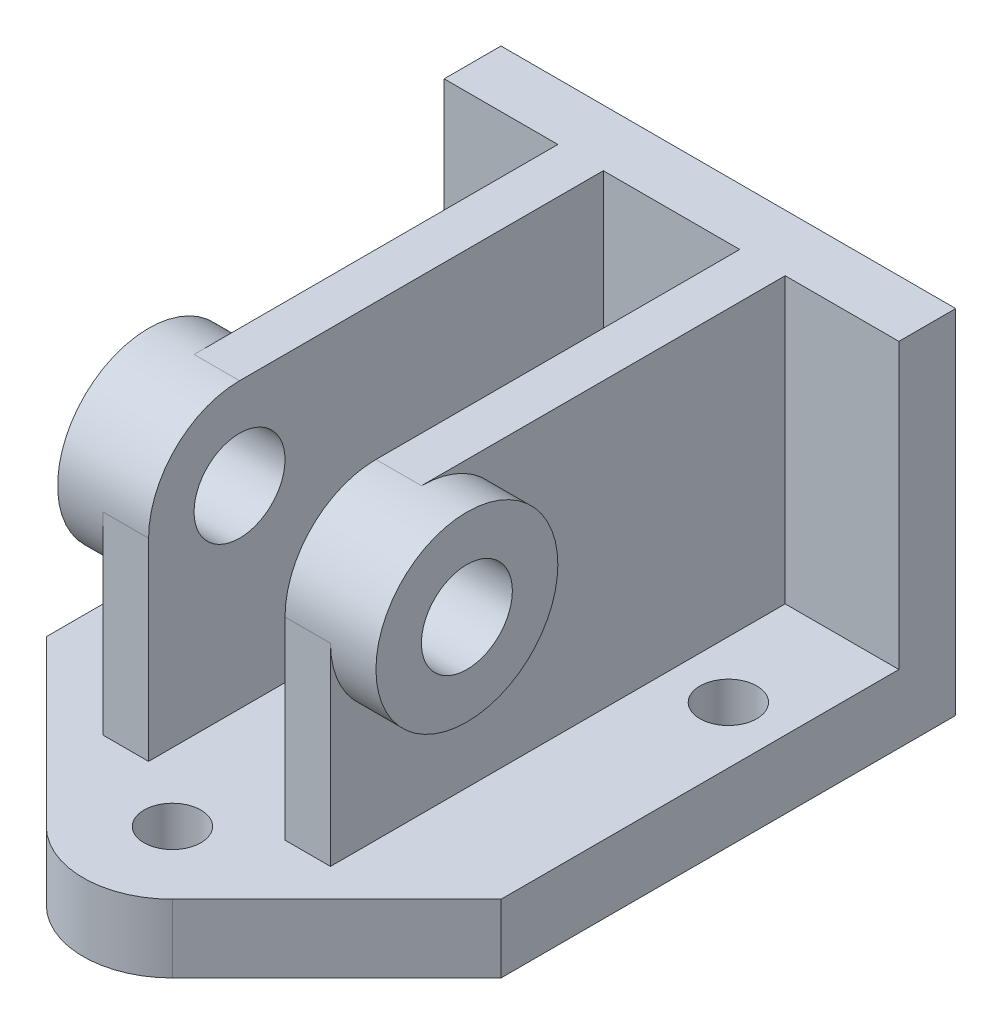
ISO-10303-21;
HEADER;
FILE_DESCRIPTION(('STEP AP214'),'2;1');
FILE_NAME('part.step','',(''),(''),'','','');
FILE_SCHEMA(('AUTOMOTIVE_DESIGN { 1 0 10303 214 1 1 1 1 }'));
ENDSEC;
DATA;
#1=APPLICATION_CONTEXT('core data for automotive mechanical design processes');
#2=APPLICATION_PROTOCOL_DEFINITION('international standard','automotive_design',2000,#1);
#3=PRODUCT_CONTEXT('',#1,'mechanical');
#4=PRODUCT('Part','Part','',(#3));
#5=PRODUCT_RELATED_PRODUCT_CATEGORY('part','',(#4));
#6=PRODUCT_DEFINITION_FORMATION('','',#4);
#7=PRODUCT_DEFINITION_CONTEXT('part definition',#1,'design');
#8=PRODUCT_DEFINITION('design','',#6,#7);
#9=PRODUCT_DEFINITION_SHAPE('','',#8);
#10=(LENGTH_UNIT() NAMED_UNIT(*) SI_UNIT(.MILLI.,.METRE.));
#11=(NAMED_UNIT(*) PLANE_ANGLE_UNIT() SI_UNIT($,.RADIAN.));
#12=(NAMED_UNIT(*) SI_UNIT($,.STERADIAN.) SOLID_ANGLE_UNIT());
#13=UNCERTAINTY_MEASURE_WITH_UNIT(LENGTH_MEASURE(1.E-05),#10,'distance_accuracy_value','');
#14=(GEOMETRIC_REPRESENTATION_CONTEXT(3) GLOBAL_UNCERTAINTY_ASSIGNED_CONTEXT((#13)) GLOBAL_UNIT_ASSIGNED_CONTEXT((#10,
#11,#12)) REPRESENTATION_CONTEXT('',''));
#15=CARTESIAN_POINT('',(0.,0.,0.));
#16=DIRECTION('',(0.,0.,1.));
#17=DIRECTION('',(1.,0.,0.));
#18=AXIS2_PLACEMENT_3D('',#15,#16,#17);
#19=CARTESIAN_POINT('',(-6.,31.,5.));
#20=DIRECTION('',(-1.,0.,0.));
#21=DIRECTION('',(0.,0.,1.));
#22=AXIS2_PLACEMENT_3D('',#19,#20,#21);
#23=PLANE('',#22);
#24=DIRECTION('',(0.,0.,-1.));
#25=VECTOR('',#24,1.);
#26=CARTESIAN_POINT('',(-6.,31.,5.));
#27=LINE('',#26,#25);
#28=CARTESIAN_POINT('',(-5.99999999999999,31.,37.));
#29=VERTEX_POINT('',#28);
#30=CARTESIAN_POINT('',(-6.,31.,5.));
#31=VERTEX_POINT('',#30);
#32=EDGE_CURVE('E289',#29,#31,#27,.T.);
#33=ORIENTED_EDGE('',*,*,#32,.F.);
#34=CARTESIAN_POINT('',(-5.99999999999999,23.,37.));
#35=DIRECTION('',(-1.,0.,0.));
#36=DIRECTION('',(0.,0.,1.));
#37=AXIS2_PLACEMENT_3D('',#34,#35,#36);
#38=CIRCLE('',#37,7.99999999999999);
#39=CARTESIAN_POINT('',(-5.99999999999999,23.,45.));
#40=VERTEX_POINT('',#39);
#41=EDGE_CURVE('E172',#29,#40,#38,.F.);
#42=ORIENTED_EDGE('',*,*,#41,.T.);
#43=DIRECTION('',(0.,-1.,0.));
#44=VECTOR('',#43,1.);
#45=CARTESIAN_POINT('',(-5.99999999999999,31.,45.));
#46=LINE('',#45,#44);
#47=CARTESIAN_POINT('',(-5.99999999999999,6.,45.));
#48=VERTEX_POINT('',#47);
#49=EDGE_CURVE('E168',#40,#48,#46,.T.);
#50=ORIENTED_EDGE('',*,*,#49,.T.);
#51=DIRECTION('',(0.,0.,-1.));
#52=VECTOR('',#51,1.);
#53=CARTESIAN_POINT('',(-6.,6.,5.));
#54=LINE('',#53,#52);
#55=CARTESIAN_POINT('',(-6.,6.,5.));
#56=VERTEX_POINT('',#55);
#57=EDGE_CURVE('E306',#48,#56,#54,.T.);
#58=ORIENTED_EDGE('',*,*,#57,.T.);
#59=DIRECTION('',(0.,-1.,0.));
#60=VECTOR('',#59,1.);
#61=CARTESIAN_POINT('',(-6.,31.,5.));
#62=LINE('',#61,#60);
#63=EDGE_CURVE('E189',#31,#56,#62,.T.);
#64=ORIENTED_EDGE('',*,*,#63,.F.);
#65=EDGE_LOOP('',(#33,#42,#50,#58,#64));
#66=FACE_BOUND('',#65,.T.);
#67=CARTESIAN_POINT('',(-5.99999999999999,23.,37.));
#68=DIRECTION('',(-1.,0.,0.));
#69=DIRECTION('',(0.,0.,1.));
#70=AXIS2_PLACEMENT_3D('',#67,#68,#69);
#71=CIRCLE('',#70,4.);
#72=CARTESIAN_POINT('',(-5.99999999999999,23.,41.));
#73=VERTEX_POINT('',#72);
#74=EDGE_CURVE('E354',#73,#73,#71,.T.);
#75=ORIENTED_EDGE('',*,*,#74,.T.);
#76=EDGE_LOOP('',(#75));
#77=FACE_BOUND('',#76,.T.);
#78=ADVANCED_FACE('F39',(#66,#77),#23,.F.);
#79=CARTESIAN_POINT('',(6.,31.,5.));
#80=DIRECTION('',(1.,0.,0.));
#81=DIRECTION('',(0.,0.,-1.));
#82=AXIS2_PLACEMENT_3D('',#79,#80,#81);
#83=PLANE('',#82);
#84=CARTESIAN_POINT('',(6.00000000000001,23.,37.));
#85=DIRECTION('',(1.,0.,0.));
#86=DIRECTION('',(0.,0.,-1.));
#87=AXIS2_PLACEMENT_3D('',#84,#85,#86);
#88=CIRCLE('',#87,7.99999999999999);
#89=CARTESIAN_POINT('',(6.,31.,37.));
#90=VERTEX_POINT('',#89);
#91=CARTESIAN_POINT('',(6.00000000000001,23.,45.));
#92=VERTEX_POINT('',#91);
#93=EDGE_CURVE('E349',#90,#92,#88,.T.);
#94=ORIENTED_EDGE('',*,*,#93,.F.);
#95=DIRECTION('',(0.,0.,1.));
#96=VECTOR('',#95,1.);
#97=CARTESIAN_POINT('',(6.,31.,5.));
#98=LINE('',#97,#96);
#99=CARTESIAN_POINT('',(6.,31.,5.));
#100=VERTEX_POINT('',#99);
#101=EDGE_CURVE('E295',#100,#90,#98,.T.);
#102=ORIENTED_EDGE('',*,*,#101,.F.);
#103=DIRECTION('',(0.,-1.,0.));
#104=VECTOR('',#103,1.);
#105=CARTESIAN_POINT('',(6.,31.,5.));
#106=LINE('',#105,#104);
#107=CARTESIAN_POINT('',(6.,6.,5.));
#108=VERTEX_POINT('',#107);
#109=EDGE_CURVE('E329',#100,#108,#106,.T.);
#110=ORIENTED_EDGE('',*,*,#109,.T.);
#111=DIRECTION('',(0.,0.,1.));
#112=VECTOR('',#111,1.);
#113=CARTESIAN_POINT('',(6.,6.,5.));
#114=LINE('',#113,#112);
#115=CARTESIAN_POINT('',(6.,6.,45.));
#116=VERTEX_POINT('',#115);
#117=EDGE_CURVE('E314',#108,#116,#114,.T.);
#118=ORIENTED_EDGE('',*,*,#117,.T.);
#119=DIRECTION('',(0.,-1.,0.));
#120=VECTOR('',#119,1.);
#121=CARTESIAN_POINT('',(6.,31.,45.));
#122=LINE('',#121,#120);
#123=EDGE_CURVE('E327',#92,#116,#122,.T.);
#124=ORIENTED_EDGE('',*,*,#123,.F.);
#125=EDGE_LOOP('',(#94,#102,#110,#118,#124));
#126=FACE_BOUND('',#125,.T.);
#127=CARTESIAN_POINT('',(6.00000000000001,23.,37.));
#128=DIRECTION('',(1.,0.,0.));
#129=DIRECTION('',(0.,0.,-1.));
#130=AXIS2_PLACEMENT_3D('',#127,#128,#129);
#131=CIRCLE('',#130,4.);
#132=CARTESIAN_POINT('',(6.00000000000001,23.,33.));
#133=VERTEX_POINT('',#132);
#134=EDGE_CURVE('E365',#133,#133,#131,.F.);
#135=ORIENTED_EDGE('',*,*,#134,.F.);
#136=EDGE_LOOP('',(#135));
#137=FACE_BOUND('',#136,.T.);
#138=ADVANCED_FACE('F347',(#126,#137),#83,.F.);
#139=CARTESIAN_POINT('',(6.,31.,45.));
#140=DIRECTION('',(0.,0.,-1.));
#141=DIRECTION('',(-1.,0.,0.));
#142=AXIS2_PLACEMENT_3D('',#139,#140,#141);
#143=PLANE('',#142);
#144=DIRECTION('',(1.,0.,0.));
#145=VECTOR('',#144,1.);
#146=CARTESIAN_POINT('',(-20.001,23.,45.));
#147=LINE('',#146,#145);
#148=CARTESIAN_POINT('',(10.,23.,45.));
#149=VERTEX_POINT('',#148);
#150=EDGE_CURVE('E369',#92,#149,#147,.T.);
#151=ORIENTED_EDGE('',*,*,#150,.F.);
#152=ORIENTED_EDGE('',*,*,#123,.T.);
#153=DIRECTION('',(1.,0.,0.));
#154=VECTOR('',#153,1.);
#155=CARTESIAN_POINT('',(6.,6.,45.));
#156=LINE('',#155,#154);
#157=CARTESIAN_POINT('',(10.,6.,45.));
#158=VERTEX_POINT('',#157);
#159=EDGE_CURVE('E320',#116,#158,#156,.T.);
#160=ORIENTED_EDGE('',*,*,#159,.T.);
#161=DIRECTION('',(0.,-1.,0.));
#162=VECTOR('',#161,1.);
#163=CARTESIAN_POINT('',(10.,31.,45.));
#164=LINE('',#163,#162);
#165=EDGE_CURVE('E326',#149,#158,#164,.T.);
#166=ORIENTED_EDGE('',*,*,#165,.F.);
#167=EDGE_LOOP('',(#151,#152,#160,#166));
#168=FACE_BOUND('',#167,.T.);
#169=ADVANCED_FACE('F390',(#168),#143,.F.);
#170=CARTESIAN_POINT('',(0.,31.,0.));
#171=DIRECTION('',(0.,1.,0.));
#172=DIRECTION('',(0.,0.,1.));
#173=AXIS2_PLACEMENT_3D('',#170,#171,#172);
#174=PLANE('',#173);
#175=DIRECTION('',(-1.,0.,0.));
#176=VECTOR('',#175,1.);
#177=CARTESIAN_POINT('',(20.001,31.,37.));
#178=LINE('',#177,#176);
#179=CARTESIAN_POINT('',(-10.,31.,37.));
#180=VERTEX_POINT('',#179);
#181=EDGE_CURVE('E174',#29,#180,#178,.T.);
#182=ORIENTED_EDGE('',*,*,#181,.F.);
#183=ORIENTED_EDGE('',*,*,#32,.T.);
#184=DIRECTION('',(1.,0.,0.));
#185=VECTOR('',#184,1.);
#186=CARTESIAN_POINT('',(-6.,31.,5.));
#187=LINE('',#186,#185);
#188=EDGE_CURVE('E288',#31,#100,#187,.T.);
#189=ORIENTED_EDGE('',*,*,#188,.T.);
#190=ORIENTED_EDGE('',*,*,#101,.T.);
#191=DIRECTION('',(1.,0.,0.));
#192=VECTOR('',#191,1.);
#193=CARTESIAN_POINT('',(-20.001,31.,37.));
#194=LINE('',#193,#192);
#195=CARTESIAN_POINT('',(10.,31.,37.));
#196=VERTEX_POINT('',#195);
#197=EDGE_CURVE('E348',#90,#196,#194,.T.);
#198=ORIENTED_EDGE('',*,*,#197,.T.);
#199=DIRECTION('',(0.,0.,-1.));
#200=VECTOR('',#199,1.);
#201=CARTESIAN_POINT('',(10.,31.,5.));
#202=LINE('',#201,#200);
#203=CARTESIAN_POINT('',(10.,31.,5.));
#204=VERTEX_POINT('',#203);
#205=EDGE_CURVE('E293',#196,#204,#202,.T.);
#206=ORIENTED_EDGE('',*,*,#205,.T.);
#207=DIRECTION('',(1.,0.,0.));
#208=VECTOR('',#207,1.);
#209=CARTESIAN_POINT('',(10.,31.,5.));
#210=LINE('',#209,#208);
#211=CARTESIAN_POINT('',(20.,31.,5.));
#212=VERTEX_POINT('',#211);
#213=EDGE_CURVE('E299',#204,#212,#210,.T.);
#214=ORIENTED_EDGE('',*,*,#213,.T.);
#215=DIRECTION('',(0.,0.,-1.));
#216=VECTOR('',#215,1.);
#217=CARTESIAN_POINT('',(20.,31.,0.));
#218=LINE('',#217,#216);
#219=CARTESIAN_POINT('',(20.,31.,0.));
#220=VERTEX_POINT('',#219);
#221=EDGE_CURVE('E296',#212,#220,#218,.T.);
#222=ORIENTED_EDGE('',*,*,#221,.T.);
#223=DIRECTION('',(-1.,0.,0.));
#224=VECTOR('',#223,1.);
#225=CARTESIAN_POINT('',(-20.,31.,0.));
#226=LINE('',#225,#224);
#227=CARTESIAN_POINT('',(-20.,31.,0.));
#228=VERTEX_POINT('',#227);
#229=EDGE_CURVE('E276',#220,#228,#226,.T.);
#230=ORIENTED_EDGE('',*,*,#229,.T.);
#231=DIRECTION('',(0.,0.,1.));
#232=VECTOR('',#231,1.);
#233=CARTESIAN_POINT('',(-20.,31.,0.));
#234=LINE('',#233,#232);
#235=CARTESIAN_POINT('',(-20.,31.,5.));
#236=VERTEX_POINT('',#235);
#237=EDGE_CURVE('E272',#228,#236,#234,.T.);
#238=ORIENTED_EDGE('',*,*,#237,.T.);
#239=DIRECTION('',(1.,0.,0.));
#240=VECTOR('',#239,1.);
#241=CARTESIAN_POINT('',(-20.,31.,5.));
#242=LINE('',#241,#240);
#243=CARTESIAN_POINT('',(-10.,31.,5.));
#244=VERTEX_POINT('',#243);
#245=EDGE_CURVE('E267',#236,#244,#242,.T.);
#246=ORIENTED_EDGE('',*,*,#245,.T.);
#247=DIRECTION('',(0.,0.,1.));
#248=VECTOR('',#247,1.);
#249=CARTESIAN_POINT('',(-10.,31.,5.));
#250=LINE('',#249,#248);
#251=EDGE_CURVE('E275',#244,#180,#250,.T.);
#252=ORIENTED_EDGE('',*,*,#251,.T.);
#253=EDGE_LOOP('',(#182,#183,#189,#190,#198,#206,#214,#222,#230,#238,#246,#252));
#254=FACE_BOUND('',#253,.T.);
#255=ADVANCED_FACE('F277',(#254),#174,.T.);
#256=CARTESIAN_POINT('',(0.,6.,48.902665169139));
#257=DIRECTION('',(0.,1.,0.));
#258=DIRECTION('',(0.,0.,1.));
#259=AXIS2_PLACEMENT_3D('',#256,#257,#258);
#260=PLANE('',#259);
#261=CARTESIAN_POINT('',(-15.,6.,15.));
#262=DIRECTION('',(0.,1.,0.));
#263=DIRECTION('',(0.,0.,1.));
#264=AXIS2_PLACEMENT_3D('',#261,#262,#263);
#265=CIRCLE('',#264,2.5);
#266=CARTESIAN_POINT('',(-15.,6.,17.5));
#267=VERTEX_POINT('',#266);
#268=EDGE_CURVE('E653',#267,#267,#265,.T.);
#269=ORIENTED_EDGE('',*,*,#268,.F.);
#270=EDGE_LOOP('',(#269));
#271=FACE_BOUND('',#270,.T.);
#272=CARTESIAN_POINT('',(15.,6.,15.));
#273=DIRECTION('',(0.,1.,0.));
#274=DIRECTION('',(0.,0.,-1.));
#275=AXIS2_PLACEMENT_3D('',#272,#273,#274);
#276=CIRCLE('',#275,2.5);
#277=CARTESIAN_POINT('',(15.,6.,17.5));
#278=VERTEX_POINT('',#277);
#279=EDGE_CURVE('E660',#278,#278,#276,.T.);
#280=ORIENTED_EDGE('',*,*,#279,.F.);
#281=EDGE_LOOP('',(#280));
#282=FACE_BOUND('',#281,.T.);
#283=DIRECTION('',(1.,0.,0.));
#284=VECTOR('',#283,1.);
#285=CARTESIAN_POINT('',(10.,6.,5.));
#286=LINE('',#285,#284);
#287=CARTESIAN_POINT('',(10.,6.,5.));
#288=VERTEX_POINT('',#287);
#289=CARTESIAN_POINT('',(20.,6.,5.));
#290=VERTEX_POINT('',#289);
#291=EDGE_CURVE('E65',#288,#290,#286,.T.);
#292=ORIENTED_EDGE('',*,*,#291,.F.);
#293=DIRECTION('',(0.,0.,-1.));
#294=VECTOR('',#293,1.);
#295=CARTESIAN_POINT('',(10.,6.,5.));
#296=LINE('',#295,#294);
#297=EDGE_CURVE('E282',#158,#288,#296,.T.);
#298=ORIENTED_EDGE('',*,*,#297,.F.);
#299=ORIENTED_EDGE('',*,*,#159,.F.);
#300=ORIENTED_EDGE('',*,*,#117,.F.);
#301=DIRECTION('',(1.,0.,0.));
#302=VECTOR('',#301,1.);
#303=CARTESIAN_POINT('',(-6.,6.,5.));
#304=LINE('',#303,#302);
#305=EDGE_CURVE('E313',#56,#108,#304,.T.);
#306=ORIENTED_EDGE('',*,*,#305,.F.);
#307=ORIENTED_EDGE('',*,*,#57,.F.);
#308=DIRECTION('',(1.,0.,0.));
#309=VECTOR('',#308,1.);
#310=CARTESIAN_POINT('',(-9.99999999999999,6.,45.));
#311=LINE('',#310,#309);
#312=CARTESIAN_POINT('',(-9.99999999999999,6.,45.));
#313=VERTEX_POINT('',#312);
#314=EDGE_CURVE('E308',#313,#48,#311,.T.);
#315=ORIENTED_EDGE('',*,*,#314,.F.);
#316=DIRECTION('',(0.,0.,1.));
#317=VECTOR('',#316,1.);
#318=CARTESIAN_POINT('',(-10.,6.,5.));
#319=LINE('',#318,#317);
#320=CARTESIAN_POINT('',(-10.,6.,5.));
#321=VERTEX_POINT('',#320);
#322=EDGE_CURVE('E185',#321,#313,#319,.T.);
#323=ORIENTED_EDGE('',*,*,#322,.F.);
#324=DIRECTION('',(1.,0.,0.));
#325=VECTOR('',#324,1.);
#326=CARTESIAN_POINT('',(-20.,6.,5.));
#327=LINE('',#326,#325);
#328=CARTESIAN_POINT('',(-20.,6.,5.));
#329=VERTEX_POINT('',#328);
#330=EDGE_CURVE('E262',#329,#321,#327,.T.);
#331=ORIENTED_EDGE('',*,*,#330,.F.);
#332=DIRECTION('',(0.,0.,1.));
#333=VECTOR('',#332,1.);
#334=CARTESIAN_POINT('',(-20.,6.,0.));
#335=LINE('',#334,#333);
#336=CARTESIAN_POINT('',(-20.,6.,40.));
#337=VERTEX_POINT('',#336);
#338=EDGE_CURVE('E199',#329,#337,#335,.T.);
#339=ORIENTED_EDGE('',*,*,#338,.T.);
#340=DIRECTION('',(0.707106781186543,0.,0.707106781186552));
#341=VECTOR('',#340,1.);
#342=CARTESIAN_POINT('',(-20.,6.,40.));
#343=LINE('',#342,#341);
#344=CARTESIAN_POINT('',(-5.54866741543061,6.,54.4513325845696));
#345=VERTEX_POINT('',#344);
#346=EDGE_CURVE('E205',#337,#345,#343,.T.);
#347=ORIENTED_EDGE('',*,*,#346,.T.);
#348=CARTESIAN_POINT('',(0.,6.,48.902665169139));
#349=DIRECTION('',(0.,1.,0.));
#350=DIRECTION('',(0.,0.,1.));
#351=AXIS2_PLACEMENT_3D('',#348,#349,#350);
#352=CIRCLE('',#351,7.84700071199961);
#353=CARTESIAN_POINT('',(5.54866741543062,6.,54.4513325845696));
#354=VERTEX_POINT('',#353);
#355=EDGE_CURVE('E202',#345,#354,#352,.T.);
#356=ORIENTED_EDGE('',*,*,#355,.T.);
#357=DIRECTION('',(0.707106781186543,0.,-0.707106781186552));
#358=VECTOR('',#357,1.);
#359=CARTESIAN_POINT('',(5.54866741543062,6.,54.4513325845696));
#360=LINE('',#359,#358);
#361=CARTESIAN_POINT('',(20.,6.,40.));
#362=VERTEX_POINT('',#361);
#363=EDGE_CURVE('E210',#354,#362,#360,.T.);
#364=ORIENTED_EDGE('',*,*,#363,.T.);
#365=DIRECTION('',(0.,0.,-1.));
#366=VECTOR('',#365,1.);
#367=CARTESIAN_POINT('',(20.,6.,0.));
#368=LINE('',#367,#366);
#369=EDGE_CURVE('E207',#362,#290,#368,.T.);
#370=ORIENTED_EDGE('',*,*,#369,.T.);
#371=EDGE_LOOP('',(#292,#298,#299,#300,#306,#307,#315,#323,#331,#339,#347,#356,#364,#370));
#372=FACE_BOUND('',#371,.T.);
#373=CARTESIAN_POINT('',(0.,6.,48.902665169139));
#374=DIRECTION('',(0.,1.,0.));
#375=DIRECTION('',(0.,0.,1.));
#376=AXIS2_PLACEMENT_3D('',#373,#374,#375);
#377=CIRCLE('',#376,2.5);
#378=CARTESIAN_POINT('',(0.,6.,51.402665169139));
#379=VERTEX_POINT('',#378);
#380=EDGE_CURVE('E191',#379,#379,#377,.T.);
#381=ORIENTED_EDGE('',*,*,#380,.F.);
#382=EDGE_LOOP('',(#381));
#383=FACE_BOUND('',#382,.T.);
#384=ADVANCED_FACE('F261',(#271,#282,#372,#383),#260,.T.);
#385=CARTESIAN_POINT('',(0.,0.,48.902665169139));
#386=DIRECTION('',(0.,1.,0.));
#387=DIRECTION('',(0.,0.,1.));
#388=AXIS2_PLACEMENT_3D('',#385,#386,#387);
#389=PLANE('',#388);
#390=CARTESIAN_POINT('',(-15.,0.,15.));
#391=DIRECTION('',(0.,1.,0.));
#392=DIRECTION('',(0.,0.,1.));
#393=AXIS2_PLACEMENT_3D('',#390,#391,#392);
#394=CIRCLE('',#393,2.5);
#395=CARTESIAN_POINT('',(-15.,0.,17.5));
#396=VERTEX_POINT('',#395);
#397=EDGE_CURVE('E353',#396,#396,#394,.F.);
#398=ORIENTED_EDGE('',*,*,#397,.F.);
#399=EDGE_LOOP('',(#398));
#400=FACE_BOUND('',#399,.T.);
#401=CARTESIAN_POINT('',(15.,0.,15.));
#402=DIRECTION('',(0.,1.,0.));
#403=DIRECTION('',(0.,0.,1.));
#404=AXIS2_PLACEMENT_3D('',#401,#402,#403);
#405=CIRCLE('',#404,2.5);
#406=CARTESIAN_POINT('',(15.,0.,17.5));
#407=VERTEX_POINT('',#406);
#408=EDGE_CURVE('E659',#407,#407,#405,.F.);
#409=ORIENTED_EDGE('',*,*,#408,.F.);
#410=EDGE_LOOP('',(#409));
#411=FACE_BOUND('',#410,.T.);
#412=DIRECTION('',(0.,0.,1.));
#413=VECTOR('',#412,1.);
#414=CARTESIAN_POINT('',(-20.,0.,0.));
#415=LINE('',#414,#413);
#416=CARTESIAN_POINT('',(-20.,0.,0.));
#417=VERTEX_POINT('',#416);
#418=CARTESIAN_POINT('',(-20.,0.,40.));
#419=VERTEX_POINT('',#418);
#420=EDGE_CURVE('E197',#417,#419,#415,.T.);
#421=ORIENTED_EDGE('',*,*,#420,.F.);
#422=DIRECTION('',(-1.,0.,0.));
#423=VECTOR('',#422,1.);
#424=CARTESIAN_POINT('',(-20.,0.,0.));
#425=LINE('',#424,#423);
#426=CARTESIAN_POINT('',(20.,0.,0.));
#427=VERTEX_POINT('',#426);
#428=EDGE_CURVE('E201',#427,#417,#425,.T.);
#429=ORIENTED_EDGE('',*,*,#428,.F.);
#430=DIRECTION('',(0.,0.,-1.));
#431=VECTOR('',#430,1.);
#432=CARTESIAN_POINT('',(20.,0.,0.));
#433=LINE('',#432,#431);
#434=CARTESIAN_POINT('',(20.,0.,40.));
#435=VERTEX_POINT('',#434);
#436=EDGE_CURVE('E219',#435,#427,#433,.T.);
#437=ORIENTED_EDGE('',*,*,#436,.F.);
#438=DIRECTION('',(0.707106781186543,0.,-0.707106781186552));
#439=VECTOR('',#438,1.);
#440=CARTESIAN_POINT('',(5.54866741543062,0.,54.4513325845696));
#441=LINE('',#440,#439);
#442=CARTESIAN_POINT('',(5.54866741543062,0.,54.4513325845696));
#443=VERTEX_POINT('',#442);
#444=EDGE_CURVE('E217',#443,#435,#441,.T.);
#445=ORIENTED_EDGE('',*,*,#444,.F.);
#446=CARTESIAN_POINT('',(0.,0.,48.902665169139));
#447=DIRECTION('',(0.,1.,0.));
#448=DIRECTION('',(0.,0.,1.));
#449=AXIS2_PLACEMENT_3D('',#446,#447,#448);
#450=CIRCLE('',#449,7.84700071199961);
#451=CARTESIAN_POINT('',(-5.54866741543061,0.,54.4513325845696));
#452=VERTEX_POINT('',#451);
#453=EDGE_CURVE('E216',#452,#443,#450,.T.);
#454=ORIENTED_EDGE('',*,*,#453,.F.);
#455=DIRECTION('',(0.707106781186543,0.,0.707106781186552));
#456=VECTOR('',#455,1.);
#457=CARTESIAN_POINT('',(-20.,0.,40.));
#458=LINE('',#457,#456);
#459=EDGE_CURVE('E212',#419,#452,#458,.T.);
#460=ORIENTED_EDGE('',*,*,#459,.F.);
#461=EDGE_LOOP('',(#421,#429,#437,#445,#454,#460));
#462=FACE_BOUND('',#461,.T.);
#463=CARTESIAN_POINT('',(0.,0.,48.902665169139));
#464=DIRECTION('',(0.,1.,0.));
#465=DIRECTION('',(0.,0.,1.));
#466=AXIS2_PLACEMENT_3D('',#463,#464,#465);
#467=CIRCLE('',#466,2.5);
#468=CARTESIAN_POINT('',(0.,0.,51.402665169139));
#469=VERTEX_POINT('',#468);
#470=EDGE_CURVE('E194',#469,#469,#467,.T.);
#471=ORIENTED_EDGE('',*,*,#470,.T.);
#472=EDGE_LOOP('',(#471));
#473=FACE_BOUND('',#472,.T.);
#474=ADVANCED_FACE('F248',(#400,#411,#462,#473),#389,.F.);
#475=CARTESIAN_POINT('',(-20.,6.,0.));
#476=DIRECTION('',(1.,0.,0.));
#477=DIRECTION('',(0.,0.,-1.));
#478=AXIS2_PLACEMENT_3D('',#475,#476,#477);
#479=PLANE('',#478);
#480=ORIENTED_EDGE('',*,*,#420,.T.);
#481=DIRECTION('',(0.,-1.,0.));
#482=VECTOR('',#481,1.);
#483=CARTESIAN_POINT('',(-20.,6.,40.));
#484=LINE('',#483,#482);
#485=EDGE_CURVE('E43',#337,#419,#484,.T.);
#486=ORIENTED_EDGE('',*,*,#485,.F.);
#487=ORIENTED_EDGE('',*,*,#338,.F.);
#488=DIRECTION('',(0.,-1.,0.));
#489=VECTOR('',#488,1.);
#490=CARTESIAN_POINT('',(-20.,31.,5.));
#491=LINE('',#490,#489);
#492=EDGE_CURVE('E183',#236,#329,#491,.T.);
#493=ORIENTED_EDGE('',*,*,#492,.F.);
#494=ORIENTED_EDGE('',*,*,#237,.F.);
#495=DIRECTION('',(0.,-1.,0.));
#496=VECTOR('',#495,1.);
#497=CARTESIAN_POINT('',(-20.,6.,0.));
#498=LINE('',#497,#496);
#499=EDGE_CURVE('E211',#228,#417,#498,.T.);
#500=ORIENTED_EDGE('',*,*,#499,.T.);
#501=EDGE_LOOP('',(#480,#486,#487,#493,#494,#500));
#502=FACE_BOUND('',#501,.T.);
#503=ADVANCED_FACE('F41',(#502),#479,.F.);
#504=CARTESIAN_POINT('',(-20.,6.,40.));
#505=DIRECTION('',(0.707106781186552,0.,-0.707106781186543));
#506=DIRECTION('',(-0.707106781186543,0.,-0.707106781186552));
#507=AXIS2_PLACEMENT_3D('',#504,#505,#506);
#508=PLANE('',#507);
#509=ORIENTED_EDGE('',*,*,#459,.T.);
#510=DIRECTION('',(0.,-1.,0.));
#511=VECTOR('',#510,1.);
#512=CARTESIAN_POINT('',(-5.54866741543061,6.,54.4513325845696));
#513=LINE('',#512,#511);
#514=EDGE_CURVE('E234',#345,#452,#513,.T.);
#515=ORIENTED_EDGE('',*,*,#514,.F.);
#516=ORIENTED_EDGE('',*,*,#346,.F.);
#517=ORIENTED_EDGE('',*,*,#485,.T.);
#518=EDGE_LOOP('',(#509,#515,#516,#517));
#519=FACE_BOUND('',#518,.T.);
#520=ADVANCED_FACE('F245',(#519),#508,.F.);
#521=CARTESIAN_POINT('',(0.,6.,48.902665169139));
#522=DIRECTION('',(0.,-1.,0.));
#523=DIRECTION('',(0.,0.,-1.));
#524=AXIS2_PLACEMENT_3D('',#521,#522,#523);
#525=CYLINDRICAL_SURFACE('',#524,7.84700071199961);
#526=ORIENTED_EDGE('',*,*,#453,.T.);
#527=DIRECTION('',(0.,-1.,0.));
#528=VECTOR('',#527,1.);
#529=CARTESIAN_POINT('',(5.54866741543062,6.,54.4513325845696));
#530=LINE('',#529,#528);
#531=EDGE_CURVE('E232',#354,#443,#530,.T.);
#532=ORIENTED_EDGE('',*,*,#531,.F.);
#533=ORIENTED_EDGE('',*,*,#355,.F.);
#534=ORIENTED_EDGE('',*,*,#514,.T.);
#535=EDGE_LOOP('',(#526,#532,#533,#534));
#536=FACE_BOUND('',#535,.T.);
#537=ADVANCED_FACE('F254',(#536),#525,.T.);
#538=CARTESIAN_POINT('',(5.54866741543062,6.,54.4513325845696));
#539=DIRECTION('',(-0.707106781186552,0.,-0.707106781186543));
#540=DIRECTION('',(-0.707106781186543,0.,0.707106781186552));
#541=AXIS2_PLACEMENT_3D('',#538,#539,#540);
#542=PLANE('',#541);
#543=ORIENTED_EDGE('',*,*,#444,.T.);
#544=DIRECTION('',(0.,-1.,0.));
#545=VECTOR('',#544,1.);
#546=CARTESIAN_POINT('',(20.,6.,40.));
#547=LINE('',#546,#545);
#548=EDGE_CURVE('E230',#362,#435,#547,.T.);
#549=ORIENTED_EDGE('',*,*,#548,.F.);
#550=ORIENTED_EDGE('',*,*,#363,.F.);
#551=ORIENTED_EDGE('',*,*,#531,.T.);
#552=EDGE_LOOP('',(#543,#549,#550,#551));
#553=FACE_BOUND('',#552,.T.);
#554=ADVANCED_FACE('F256',(#553),#542,.F.);
#555=CARTESIAN_POINT('',(20.,6.,0.));
#556=DIRECTION('',(-1.,0.,0.));
#557=DIRECTION('',(0.,0.,1.));
#558=AXIS2_PLACEMENT_3D('',#555,#556,#557);
#559=PLANE('',#558);
#560=ORIENTED_EDGE('',*,*,#436,.T.);
#561=DIRECTION('',(0.,-1.,0.));
#562=VECTOR('',#561,1.);
#563=CARTESIAN_POINT('',(20.,6.,0.));
#564=LINE('',#563,#562);
#565=EDGE_CURVE('E223',#220,#427,#564,.T.);
#566=ORIENTED_EDGE('',*,*,#565,.F.);
#567=ORIENTED_EDGE('',*,*,#221,.F.);
#568=DIRECTION('',(0.,-1.,0.));
#569=VECTOR('',#568,1.);
#570=CARTESIAN_POINT('',(20.,31.,5.));
#571=LINE('',#570,#569);
#572=EDGE_CURVE('E305',#212,#290,#571,.T.);
#573=ORIENTED_EDGE('',*,*,#572,.T.);
#574=ORIENTED_EDGE('',*,*,#369,.F.);
#575=ORIENTED_EDGE('',*,*,#548,.T.);
#576=EDGE_LOOP('',(#560,#566,#567,#573,#574,#575));
#577=FACE_BOUND('',#576,.T.);
#578=ADVANCED_FACE('F424',(#577),#559,.F.);
#579=CARTESIAN_POINT('',(-20.,6.,0.));
#580=DIRECTION('',(0.,0.,1.));
#581=DIRECTION('',(1.,0.,0.));
#582=AXIS2_PLACEMENT_3D('',#579,#580,#581);
#583=PLANE('',#582);
#584=ORIENTED_EDGE('',*,*,#428,.T.);
#585=ORIENTED_EDGE('',*,*,#499,.F.);
#586=ORIENTED_EDGE('',*,*,#229,.F.);
#587=ORIENTED_EDGE('',*,*,#565,.T.);
#588=EDGE_LOOP('',(#584,#585,#586,#587));
#589=FACE_BOUND('',#588,.T.);
#590=ADVANCED_FACE('F411',(#589),#583,.F.);
#591=CARTESIAN_POINT('',(0.,6.,48.902665169139));
#592=DIRECTION('',(0.,-1.,0.));
#593=DIRECTION('',(0.,0.,-1.));
#594=AXIS2_PLACEMENT_3D('',#591,#592,#593);
#595=CYLINDRICAL_SURFACE('',#594,2.5);
#596=ORIENTED_EDGE('',*,*,#380,.T.);
#597=EDGE_LOOP('',(#596));
#598=FACE_BOUND('',#597,.T.);
#599=ORIENTED_EDGE('',*,*,#470,.F.);
#600=EDGE_LOOP('',(#599));
#601=FACE_BOUND('',#600,.T.);
#602=ADVANCED_FACE('F412',(#598,#601),#595,.F.);
#603=CARTESIAN_POINT('',(-20.,31.,5.));
#604=DIRECTION('',(0.,0.,-1.));
#605=DIRECTION('',(-1.,0.,0.));
#606=AXIS2_PLACEMENT_3D('',#603,#604,#605);
#607=PLANE('',#606);
#608=ORIENTED_EDGE('',*,*,#330,.T.);
#609=DIRECTION('',(0.,-1.,0.));
#610=VECTOR('',#609,1.);
#611=CARTESIAN_POINT('',(-10.,31.,5.));
#612=LINE('',#611,#610);
#613=EDGE_CURVE('E181',#244,#321,#612,.T.);
#614=ORIENTED_EDGE('',*,*,#613,.F.);
#615=ORIENTED_EDGE('',*,*,#245,.F.);
#616=ORIENTED_EDGE('',*,*,#492,.T.);
#617=EDGE_LOOP('',(#608,#614,#615,#616));
#618=FACE_BOUND('',#617,.T.);
#619=ADVANCED_FACE('F270',(#618),#607,.F.);
#620=CARTESIAN_POINT('',(-10.,31.,5.));
#621=DIRECTION('',(1.,0.,0.));
#622=DIRECTION('',(0.,0.,-1.));
#623=AXIS2_PLACEMENT_3D('',#620,#621,#622);
#624=PLANE('',#623);
#625=DIRECTION('',(0.,-1.,0.));
#626=VECTOR('',#625,1.);
#627=CARTESIAN_POINT('',(-9.99999999999999,31.,45.));
#628=LINE('',#627,#626);
#629=CARTESIAN_POINT('',(-10.,23.,45.));
#630=VERTEX_POINT('',#629);
#631=EDGE_CURVE('E169',#630,#313,#628,.T.);
#632=ORIENTED_EDGE('',*,*,#631,.F.);
#633=CARTESIAN_POINT('',(-10.,23.,37.));
#634=DIRECTION('',(1.,0.,0.));
#635=DIRECTION('',(0.,0.,-1.));
#636=AXIS2_PLACEMENT_3D('',#633,#634,#635);
#637=CIRCLE('',#636,8.);
#638=EDGE_CURVE('E11',#630,#180,#637,.T.);
#639=ORIENTED_EDGE('',*,*,#638,.T.);
#640=ORIENTED_EDGE('',*,*,#251,.F.);
#641=ORIENTED_EDGE('',*,*,#613,.T.);
#642=ORIENTED_EDGE('',*,*,#322,.T.);
#643=EDGE_LOOP('',(#632,#639,#640,#641,#642));
#644=FACE_BOUND('',#643,.T.);
#645=ADVANCED_FACE('F178',(#644),#624,.F.);
#646=CARTESIAN_POINT('',(-9.99999999999999,31.,45.));
#647=DIRECTION('',(0.,0.,-1.));
#648=DIRECTION('',(-1.,0.,0.));
#649=AXIS2_PLACEMENT_3D('',#646,#647,#648);
#650=PLANE('',#649);
#651=ORIENTED_EDGE('',*,*,#49,.F.);
#652=DIRECTION('',(-1.,0.,0.));
#653=VECTOR('',#652,1.);
#654=CARTESIAN_POINT('',(20.001,23.,45.));
#655=LINE('',#654,#653);
#656=EDGE_CURVE('E54',#40,#630,#655,.T.);
#657=ORIENTED_EDGE('',*,*,#656,.T.);
#658=ORIENTED_EDGE('',*,*,#631,.T.);
#659=ORIENTED_EDGE('',*,*,#314,.T.);
#660=EDGE_LOOP('',(#651,#657,#658,#659));
#661=FACE_BOUND('',#660,.T.);
#662=ADVANCED_FACE('F164',(#661),#650,.F.);
#663=CARTESIAN_POINT('',(-6.,31.,5.));
#664=DIRECTION('',(0.,0.,-1.));
#665=DIRECTION('',(-1.,0.,0.));
#666=AXIS2_PLACEMENT_3D('',#663,#664,#665);
#667=PLANE('',#666);
#668=ORIENTED_EDGE('',*,*,#305,.T.);
#669=ORIENTED_EDGE('',*,*,#109,.F.);
#670=ORIENTED_EDGE('',*,*,#188,.F.);
#671=ORIENTED_EDGE('',*,*,#63,.T.);
#672=EDGE_LOOP('',(#668,#669,#670,#671));
#673=FACE_BOUND('',#672,.T.);
#674=ADVANCED_FACE('F337',(#673),#667,.F.);
#675=CARTESIAN_POINT('',(10.,31.,5.));
#676=DIRECTION('',(-1.,0.,0.));
#677=DIRECTION('',(0.,0.,1.));
#678=AXIS2_PLACEMENT_3D('',#675,#676,#677);
#679=PLANE('',#678);
#680=CARTESIAN_POINT('',(10.,23.,37.));
#681=DIRECTION('',(1.,0.,0.));
#682=DIRECTION('',(0.,0.,-1.));
#683=AXIS2_PLACEMENT_3D('',#680,#681,#682);
#684=CIRCLE('',#683,8.);
#685=EDGE_CURVE('E281',#149,#196,#684,.T.);
#686=ORIENTED_EDGE('',*,*,#685,.F.);
#687=ORIENTED_EDGE('',*,*,#165,.T.);
#688=ORIENTED_EDGE('',*,*,#297,.T.);
#689=DIRECTION('',(0.,-1.,0.));
#690=VECTOR('',#689,1.);
#691=CARTESIAN_POINT('',(10.,31.,5.));
#692=LINE('',#691,#690);
#693=EDGE_CURVE('E323',#204,#288,#692,.T.);
#694=ORIENTED_EDGE('',*,*,#693,.F.);
#695=ORIENTED_EDGE('',*,*,#205,.F.);
#696=EDGE_LOOP('',(#686,#687,#688,#694,#695));
#697=FACE_BOUND('',#696,.T.);
#698=ADVANCED_FACE('F383',(#697),#679,.F.);
#699=CARTESIAN_POINT('',(10.,31.,5.));
#700=DIRECTION('',(0.,0.,-1.));
#701=DIRECTION('',(-1.,0.,0.));
#702=AXIS2_PLACEMENT_3D('',#699,#700,#701);
#703=PLANE('',#702);
#704=ORIENTED_EDGE('',*,*,#291,.T.);
#705=ORIENTED_EDGE('',*,*,#572,.F.);
#706=ORIENTED_EDGE('',*,*,#213,.F.);
#707=ORIENTED_EDGE('',*,*,#693,.T.);
#708=EDGE_LOOP('',(#704,#705,#706,#707));
#709=FACE_BOUND('',#708,.T.);
#710=ADVANCED_FACE('F469',(#709),#703,.F.);
#711=CARTESIAN_POINT('',(14.,23.,37.));
#712=DIRECTION('',(1.,0.,0.));
#713=DIRECTION('',(0.,0.,-1.));
#714=AXIS2_PLACEMENT_3D('',#711,#712,#713);
#715=PLANE('',#714);
#716=CARTESIAN_POINT('',(14.,23.,37.));
#717=DIRECTION('',(1.,0.,0.));
#718=DIRECTION('',(0.,0.,-1.));
#719=AXIS2_PLACEMENT_3D('',#716,#717,#718);
#720=CIRCLE('',#719,8.);
#721=CARTESIAN_POINT('',(14.,23.,29.));
#722=VERTEX_POINT('',#721);
#723=EDGE_CURVE('E301',#722,#722,#720,.T.);
#724=ORIENTED_EDGE('',*,*,#723,.T.);
#725=EDGE_LOOP('',(#724));
#726=FACE_BOUND('',#725,.T.);
#727=CARTESIAN_POINT('',(14.,23.,37.));
#728=DIRECTION('',(1.,0.,0.));
#729=DIRECTION('',(0.,0.,-1.));
#730=AXIS2_PLACEMENT_3D('',#727,#728,#729);
#731=CIRCLE('',#730,4.);
#732=CARTESIAN_POINT('',(14.,23.,33.));
#733=VERTEX_POINT('',#732);
#734=EDGE_CURVE('E371',#733,#733,#731,.T.);
#735=ORIENTED_EDGE('',*,*,#734,.F.);
#736=EDGE_LOOP('',(#735));
#737=FACE_BOUND('',#736,.T.);
#738=ADVANCED_FACE('F472',(#726,#737),#715,.T.);
#739=CARTESIAN_POINT('',(14.,23.,37.));
#740=DIRECTION('',(-1.,0.,0.));
#741=DIRECTION('',(0.,0.,1.));
#742=AXIS2_PLACEMENT_3D('',#739,#740,#741);
#743=CYLINDRICAL_SURFACE('',#742,8.);
#744=ORIENTED_EDGE('',*,*,#723,.F.);
#745=EDGE_LOOP('',(#744));
#746=FACE_BOUND('',#745,.T.);
#747=ORIENTED_EDGE('',*,*,#685,.T.);
#748=ORIENTED_EDGE('',*,*,#197,.F.);
#749=ORIENTED_EDGE('',*,*,#93,.T.);
#750=ORIENTED_EDGE('',*,*,#150,.T.);
#751=EDGE_LOOP('',(#747,#748,#749,#750));
#752=FACE_BOUND('',#751,.T.);
#753=ADVANCED_FACE('F379',(#746,#752),#743,.T.);
#754=CARTESIAN_POINT('',(14.,23.,37.));
#755=DIRECTION('',(-1.,0.,0.));
#756=DIRECTION('',(0.,0.,1.));
#757=AXIS2_PLACEMENT_3D('',#754,#755,#756);
#758=CYLINDRICAL_SURFACE('',#757,4.);
#759=ORIENTED_EDGE('',*,*,#734,.T.);
#760=EDGE_LOOP('',(#759));
#761=FACE_BOUND('',#760,.T.);
#762=ORIENTED_EDGE('',*,*,#134,.T.);
#763=EDGE_LOOP('',(#762));
#764=FACE_BOUND('',#763,.T.);
#765=ADVANCED_FACE('F502',(#761,#764),#758,.F.);
#766=CARTESIAN_POINT('',(-14.,23.,37.));
#767=DIRECTION('',(1.,0.,0.));
#768=DIRECTION('',(0.,0.,-1.));
#769=AXIS2_PLACEMENT_3D('',#766,#767,#768);
#770=CYLINDRICAL_SURFACE('',#769,8.);
#771=CARTESIAN_POINT('',(-14.,23.,37.));
#772=DIRECTION('',(1.,0.,0.));
#773=DIRECTION('',(0.,0.,-1.));
#774=AXIS2_PLACEMENT_3D('',#771,#772,#773);
#775=CIRCLE('',#774,8.);
#776=CARTESIAN_POINT('',(-14.,23.,29.));
#777=VERTEX_POINT('',#776);
#778=EDGE_CURVE('E362',#777,#777,#775,.T.);
#779=ORIENTED_EDGE('',*,*,#778,.T.);
#780=EDGE_LOOP('',(#779));
#781=FACE_BOUND('',#780,.T.);
#782=ORIENTED_EDGE('',*,*,#638,.F.);
#783=ORIENTED_EDGE('',*,*,#656,.F.);
#784=ORIENTED_EDGE('',*,*,#41,.F.);
#785=ORIENTED_EDGE('',*,*,#181,.T.);
#786=EDGE_LOOP('',(#782,#783,#784,#785));
#787=FACE_BOUND('',#786,.T.);
#788=ADVANCED_FACE('F171',(#781,#787),#770,.T.);
#789=CARTESIAN_POINT('',(-14.,23.,37.));
#790=DIRECTION('',(-1.,0.,0.));
#791=DIRECTION('',(0.,0.,-1.));
#792=AXIS2_PLACEMENT_3D('',#789,#790,#791);
#793=PLANE('',#792);
#794=CARTESIAN_POINT('',(-14.,23.,37.));
#795=DIRECTION('',(1.,0.,0.));
#796=DIRECTION('',(0.,0.,-1.));
#797=AXIS2_PLACEMENT_3D('',#794,#795,#796);
#798=CIRCLE('',#797,4.);
#799=CARTESIAN_POINT('',(-14.,23.,33.));
#800=VERTEX_POINT('',#799);
#801=EDGE_CURVE('E356',#800,#800,#798,.T.);
#802=ORIENTED_EDGE('',*,*,#801,.T.);
#803=EDGE_LOOP('',(#802));
#804=FACE_BOUND('',#803,.T.);
#805=ORIENTED_EDGE('',*,*,#778,.F.);
#806=EDGE_LOOP('',(#805));
#807=FACE_BOUND('',#806,.T.);
#808=ADVANCED_FACE('F498',(#804,#807),#793,.T.);
#809=CARTESIAN_POINT('',(-14.,23.,37.));
#810=DIRECTION('',(1.,0.,0.));
#811=DIRECTION('',(0.,0.,-1.));
#812=AXIS2_PLACEMENT_3D('',#809,#810,#811);
#813=CYLINDRICAL_SURFACE('',#812,4.);
#814=ORIENTED_EDGE('',*,*,#801,.F.);
#815=EDGE_LOOP('',(#814));
#816=FACE_BOUND('',#815,.T.);
#817=ORIENTED_EDGE('',*,*,#74,.F.);
#818=EDGE_LOOP('',(#817));
#819=FACE_BOUND('',#818,.T.);
#820=ADVANCED_FACE('F515',(#816,#819),#813,.F.);
#821=CARTESIAN_POINT('',(15.,-0.00100000000000013,15.));
#822=DIRECTION('',(0.,1.,0.));
#823=DIRECTION('',(0.,0.,1.));
#824=AXIS2_PLACEMENT_3D('',#821,#822,#823);
#825=CYLINDRICAL_SURFACE('',#824,2.5);
#826=CARTESIAN_POINT('',(15.,6.,17.5));
#827=CARTESIAN_POINT('',(15.,5.9375,17.5));
#828=CARTESIAN_POINT('',(15.,5.875,17.5));
#829=CARTESIAN_POINT('',(15.,5.75,17.5));
#830=CARTESIAN_POINT('',(15.,5.6875,17.5));
#831=CARTESIAN_POINT('',(15.,5.5625,17.5));
#832=CARTESIAN_POINT('',(15.,5.5,17.5));
#833=CARTESIAN_POINT('',(15.,5.375,17.5));
#834=CARTESIAN_POINT('',(15.,5.3125,17.5));
#835=CARTESIAN_POINT('',(15.,5.1875,17.5));
#836=CARTESIAN_POINT('',(15.,5.125,17.5));
#837=CARTESIAN_POINT('',(15.,5.,17.5));
#838=CARTESIAN_POINT('',(15.,4.9375,17.5));
#839=CARTESIAN_POINT('',(15.,4.8125,17.5));
#840=CARTESIAN_POINT('',(15.,4.75,17.5));
#841=CARTESIAN_POINT('',(15.,4.625,17.5));
#842=CARTESIAN_POINT('',(15.,4.5625,17.5));
#843=CARTESIAN_POINT('',(15.,4.4375,17.5));
#844=CARTESIAN_POINT('',(15.,4.375,17.5));
#845=CARTESIAN_POINT('',(15.,4.25,17.5));
#846=CARTESIAN_POINT('',(15.,4.1875,17.5));
#847=CARTESIAN_POINT('',(15.,4.0625,17.5));
#848=CARTESIAN_POINT('',(15.,4.,17.5));
#849=CARTESIAN_POINT('',(15.,3.875,17.5));
#850=CARTESIAN_POINT('',(15.,3.8125,17.5));
#851=CARTESIAN_POINT('',(15.,3.6875,17.5));
#852=CARTESIAN_POINT('',(15.,3.625,17.5));
#853=CARTESIAN_POINT('',(15.,3.5,17.5));
#854=CARTESIAN_POINT('',(15.,3.4375,17.5));
#855=CARTESIAN_POINT('',(15.,3.3125,17.5));
#856=CARTESIAN_POINT('',(15.,3.25,17.5));
#857=CARTESIAN_POINT('',(15.,3.125,17.5));
#858=CARTESIAN_POINT('',(15.,3.0625,17.5));
#859=CARTESIAN_POINT('',(15.,2.9375,17.5));
#860=CARTESIAN_POINT('',(15.,2.875,17.5));
#861=CARTESIAN_POINT('',(15.,2.75,17.5));
#862=CARTESIAN_POINT('',(15.,2.6875,17.5));
#863=CARTESIAN_POINT('',(15.,2.5625,17.5));
#864=CARTESIAN_POINT('',(15.,2.5,17.5));
#865=CARTESIAN_POINT('',(15.,2.375,17.5));
#866=CARTESIAN_POINT('',(15.,2.3125,17.5));
#867=CARTESIAN_POINT('',(15.,2.1875,17.5));
#868=CARTESIAN_POINT('',(15.,2.125,17.5));
#869=CARTESIAN_POINT('',(15.,2.,17.5));
#870=CARTESIAN_POINT('',(15.,1.9375,17.5));
#871=CARTESIAN_POINT('',(15.,1.8125,17.5));
#872=CARTESIAN_POINT('',(15.,1.75,17.5));
#873=CARTESIAN_POINT('',(15.,1.625,17.5));
#874=CARTESIAN_POINT('',(15.,1.5625,17.5));
#875=CARTESIAN_POINT('',(15.,1.4375,17.5));
#876=CARTESIAN_POINT('',(15.,1.375,17.5));
#877=CARTESIAN_POINT('',(15.,1.25,17.5));
#878=CARTESIAN_POINT('',(15.,1.1875,17.5));
#879=CARTESIAN_POINT('',(15.,1.0625,17.5));
#880=CARTESIAN_POINT('',(15.,1.,17.5));
#881=CARTESIAN_POINT('',(15.,0.875,17.5));
#882=CARTESIAN_POINT('',(15.,0.8125,17.5));
#883=CARTESIAN_POINT('',(15.,0.6875,17.5));
#884=CARTESIAN_POINT('',(15.,0.625,17.5));
#885=CARTESIAN_POINT('',(15.,0.5,17.5));
#886=CARTESIAN_POINT('',(15.,0.4375,17.5));
#887=CARTESIAN_POINT('',(15.,0.3125,17.5));
#888=CARTESIAN_POINT('',(15.,0.25,17.5));
#889=CARTESIAN_POINT('',(15.,0.125,17.5));
#890=CARTESIAN_POINT('',(15.,0.0625000000000001,17.5));
#891=CARTESIAN_POINT('',(15.,0.,17.5));
#892=B_SPLINE_CURVE_WITH_KNOTS('',3,(#826,#827,#828,#829,#830,#831,#832,#833,#834,#835,#836,
#837,#838,#839,#840,#841,#842,#843,#844,#845,#846,#847,#848,#849,#850,#851,#852,#853,#854,#855,
#856,#857,#858,#859,#860,#861,#862,#863,#864,#865,#866,#867,#868,#869,#870,#871,#872,#873,#874,
#875,#876,#877,#878,#879,#880,#881,#882,#883,#884,#885,#886,#887,#888,#889,#890,#891),
.UNSPECIFIED.,.F.,.F.,(4,2,2,2,2,2,2,2,2,2,2,2,2,2,2,2,2,2,2,2,2,2,2,2,2,2,2,2,2,2,2,2,4),(0.,
0.1875,0.375,0.5625,0.75,0.9375,1.125,1.3125,1.5,1.6875,1.875,2.0625,2.25,2.4375,2.625,2.8125,
3.,3.1875,3.375,3.5625,3.75,3.9375,4.125,4.3125,4.5,4.6875,4.875,5.0625,5.25,5.4375,5.625,
5.8125,6.),.UNSPECIFIED.);
#893=EDGE_CURVE('BSEAM518',#278,#407,#892,.T.);
#894=ORIENTED_EDGE('',*,*,#279,.T.);
#895=ORIENTED_EDGE('',*,*,#408,.T.);
#896=ORIENTED_EDGE('',*,*,#893,.T.);
#897=ORIENTED_EDGE('',*,*,#893,.F.);
#898=EDGE_LOOP('',(#894,#896,#895,#897));
#899=FACE_BOUND('',#898,.T.);
#900=ADVANCED_FACE('F518',(#899),#825,.F.);
#901=CARTESIAN_POINT('',(-15.,-0.00100000000000013,15.));
#902=DIRECTION('',(0.,1.,0.));
#903=DIRECTION('',(0.,0.,1.));
#904=AXIS2_PLACEMENT_3D('',#901,#902,#903);
#905=CYLINDRICAL_SURFACE('',#904,2.5);
#906=CARTESIAN_POINT('',(-15.,6.,17.5));
#907=CARTESIAN_POINT('',(-15.,5.9375,17.5));
#908=CARTESIAN_POINT('',(-15.,5.875,17.5));
#909=CARTESIAN_POINT('',(-15.,5.75,17.5));
#910=CARTESIAN_POINT('',(-15.,5.6875,17.5));
#911=CARTESIAN_POINT('',(-15.,5.5625,17.5));
#912=CARTESIAN_POINT('',(-15.,5.5,17.5));
#913=CARTESIAN_POINT('',(-15.,5.375,17.5));
#914=CARTESIAN_POINT('',(-15.,5.3125,17.5));
#915=CARTESIAN_POINT('',(-15.,5.1875,17.5));
#916=CARTESIAN_POINT('',(-15.,5.125,17.5));
#917=CARTESIAN_POINT('',(-15.,5.,17.5));
#918=CARTESIAN_POINT('',(-15.,4.9375,17.5));
#919=CARTESIAN_POINT('',(-15.,4.8125,17.5));
#920=CARTESIAN_POINT('',(-15.,4.75,17.5));
#921=CARTESIAN_POINT('',(-15.,4.625,17.5));
#922=CARTESIAN_POINT('',(-15.,4.5625,17.5));
#923=CARTESIAN_POINT('',(-15.,4.4375,17.5));
#924=CARTESIAN_POINT('',(-15.,4.375,17.5));
#925=CARTESIAN_POINT('',(-15.,4.25,17.5));
#926=CARTESIAN_POINT('',(-15.,4.1875,17.5));
#927=CARTESIAN_POINT('',(-15.,4.0625,17.5));
#928=CARTESIAN_POINT('',(-15.,4.,17.5));
#929=CARTESIAN_POINT('',(-15.,3.875,17.5));
#930=CARTESIAN_POINT('',(-15.,3.8125,17.5));
#931=CARTESIAN_POINT('',(-15.,3.6875,17.5));
#932=CARTESIAN_POINT('',(-15.,3.625,17.5));
#933=CARTESIAN_POINT('',(-15.,3.5,17.5));
#934=CARTESIAN_POINT('',(-15.,3.4375,17.5));
#935=CARTESIAN_POINT('',(-15.,3.3125,17.5));
#936=CARTESIAN_POINT('',(-15.,3.25,17.5));
#937=CARTESIAN_POINT('',(-15.,3.125,17.5));
#938=CARTESIAN_POINT('',(-15.,3.0625,17.5));
#939=CARTESIAN_POINT('',(-15.,2.9375,17.5));
#940=CARTESIAN_POINT('',(-15.,2.875,17.5));
#941=CARTESIAN_POINT('',(-15.,2.75,17.5));
#942=CARTESIAN_POINT('',(-15.,2.6875,17.5));
#943=CARTESIAN_POINT('',(-15.,2.5625,17.5));
#944=CARTESIAN_POINT('',(-15.,2.5,17.5));
#945=CARTESIAN_POINT('',(-15.,2.375,17.5));
#946=CARTESIAN_POINT('',(-15.,2.3125,17.5));
#947=CARTESIAN_POINT('',(-15.,2.1875,17.5));
#948=CARTESIAN_POINT('',(-15.,2.125,17.5));
#949=CARTESIAN_POINT('',(-15.,2.,17.5));
#950=CARTESIAN_POINT('',(-15.,1.9375,17.5));
#951=CARTESIAN_POINT('',(-15.,1.8125,17.5));
#952=CARTESIAN_POINT('',(-15.,1.75,17.5));
#953=CARTESIAN_POINT('',(-15.,1.625,17.5));
#954=CARTESIAN_POINT('',(-15.,1.5625,17.5));
#955=CARTESIAN_POINT('',(-15.,1.4375,17.5));
#956=CARTESIAN_POINT('',(-15.,1.375,17.5));
#957=CARTESIAN_POINT('',(-15.,1.25,17.5));
#958=CARTESIAN_POINT('',(-15.,1.1875,17.5));
#959=CARTESIAN_POINT('',(-15.,1.0625,17.5));
#960=CARTESIAN_POINT('',(-15.,1.,17.5));
#961=CARTESIAN_POINT('',(-15.,0.875,17.5));
#962=CARTESIAN_POINT('',(-15.,0.8125,17.5));
#963=CARTESIAN_POINT('',(-15.,0.6875,17.5));
#964=CARTESIAN_POINT('',(-15.,0.625,17.5));
#965=CARTESIAN_POINT('',(-15.,0.5,17.5));
#966=CARTESIAN_POINT('',(-15.,0.4375,17.5));
#967=CARTESIAN_POINT('',(-15.,0.3125,17.5));
#968=CARTESIAN_POINT('',(-15.,0.25,17.5));
#969=CARTESIAN_POINT('',(-15.,0.125,17.5));
#970=CARTESIAN_POINT('',(-15.,0.0625000000000001,17.5));
#971=CARTESIAN_POINT('',(-15.,0.,17.5));
#972=B_SPLINE_CURVE_WITH_KNOTS('',3,(#906,#907,#908,#909,#910,#911,#912,#913,#914,#915,#916,
#917,#918,#919,#920,#921,#922,#923,#924,#925,#926,#927,#928,#929,#930,#931,#932,#933,#934,#935,
#936,#937,#938,#939,#940,#941,#942,#943,#944,#945,#946,#947,#948,#949,#950,#951,#952,#953,#954,
#955,#956,#957,#958,#959,#960,#961,#962,#963,#964,#965,#966,#967,#968,#969,#970,#971),
.UNSPECIFIED.,.F.,.F.,(4,2,2,2,2,2,2,2,2,2,2,2,2,2,2,2,2,2,2,2,2,2,2,2,2,2,2,2,2,2,2,2,4),(0.,
0.1875,0.375,0.5625,0.75,0.9375,1.125,1.3125,1.5,1.6875,1.875,2.0625,2.25,2.4375,2.625,2.8125,
3.,3.1875,3.375,3.5625,3.75,3.9375,4.125,4.3125,4.5,4.6875,4.875,5.0625,5.25,5.4375,5.625,
5.8125,6.),.UNSPECIFIED.);
#973=EDGE_CURVE('BSEAM532',#267,#396,#972,.T.);
#974=ORIENTED_EDGE('',*,*,#268,.T.);
#975=ORIENTED_EDGE('',*,*,#397,.T.);
#976=ORIENTED_EDGE('',*,*,#973,.T.);
#977=ORIENTED_EDGE('',*,*,#973,.F.);
#978=EDGE_LOOP('',(#974,#976,#975,#977));
#979=FACE_BOUND('',#978,.T.);
#980=ADVANCED_FACE('F532',(#979),#905,.F.);
#981=CLOSED_SHELL('',(#78,#138,#169,#255,#384,#474,#503,#520,#537,#554,#578,#590,#602,#619,#645,
#662,#674,#698,#710,#738,#753,#765,#788,#808,#820,#900,#980));
#982=MANIFOLD_SOLID_BREP('B2',#981);
#983=ADVANCED_BREP_SHAPE_REPRESENTATION('',(#18,#982),#14);
#984=SHAPE_DEFINITION_REPRESENTATION(#9,#983);
ENDSEC;
END-ISO-10303-21;
